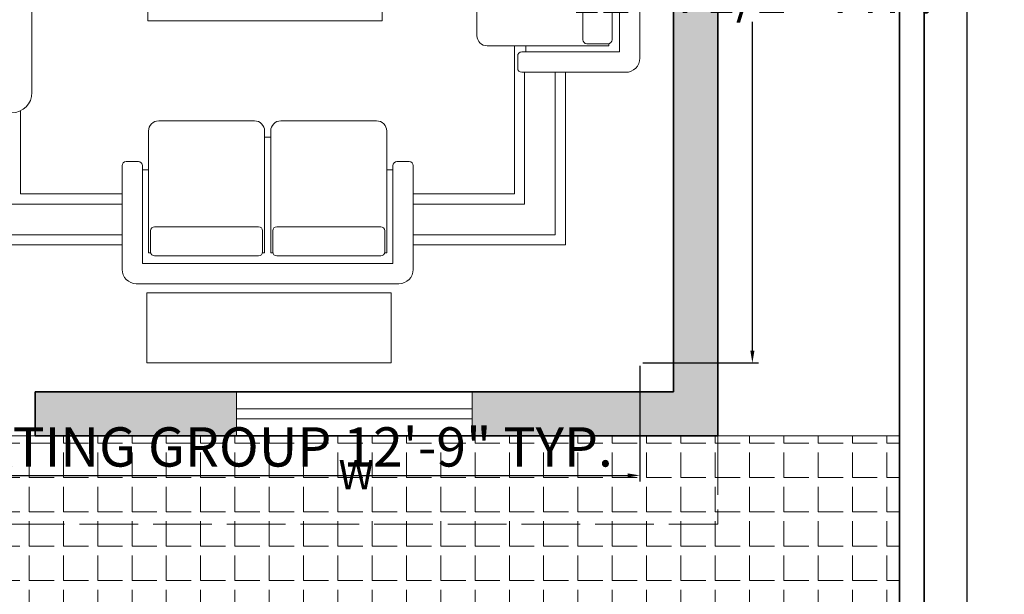
# Model space of a CAD drawing. Units: inches. Extents: x 1070 to 2371, y 645 to 1546.
# Tile 4 of 10: x 1458 to 1658, y 772 to 890. Entities that reach past the tile are written whole.
import ezdxf

# ---------------------------------------------------------------- set-up
doc = ezdxf.new("R2010")
doc.units = ezdxf.units.IN
doc.linetypes.add('ACAD_ISO02W100', pattern=[15, 12, -3])
for name, color, linetype, lineweight in [('A-ANNO-DIMS', 2, 'Continuous', 18), ('A-ANNO-TEXT', 7, 'Continuous', 18), ('A-DOOR', 4, 'Continuous', 18), ('A-FURN', 8, 'Continuous', 18), ('A-GLAZ', 4, 'Continuous', 18), ('A-ROOF-OVHD', 8, 'ACAD_ISO02W100', 13), ('A-WALL', 7, 'Continuous', 35), ('C-PROP', 7, 'Continuous', 35), ('L-PLNT-BEDS', 3, 'Continuous', 18), ('L-TURF-PATT', 9, 'Continuous', 13)]:
    doc.layers.add(name, color=color, linetype=linetype, lineweight=lineweight)
doc.layers.add('A-WALL-PATT', color=162, linetype='Continuous', lineweight=13, true_color=0x044ac3)
doc.styles.get("Standard").update_dxf_attribs({"font": 'arial.ttf'})
doc.dimstyles.new('ISO-25', dxfattribs={"dimtxt": 8, "dimasz": 2.5, "dimexe": 1.25, "dimexo": 0.625, "dimtad": 1, "dimtih": 1, "dimtoh": 1, "dimdec": 1, "dimlunit": 3, "dimtxsty": 'Standard', "dimcen": 2.5, "dimadec": 0, "dimazin": 0, "dimtfac": 1, "dimtdec": 1, "dimtmove": 0, "dimatfit": 3, "dimfxl": 1, "dimarcsym": 0})

# ---------------------------------------------------------------- blocks, each defined once
blk = doc.blocks.new('A$C71DE5BFE')
for p, q in [((2753, 3552), (893, 3552)), ((823, 3482), (823, 2972)), ((2823, 2972), (2823, 3482)), ((923, 3452), (2723, 3452)), ((923, 2972), (923, 3452)), ((2723, 3452), (2723, 2972)), ((430.7, 3295.7), (503.4, 3397.4)), ((963.5, 3399.9), (953, 3399.9)), ((953, 3399.9), (953, 2802)), ((963, 3292), (963, 3395.7)), ((1493, 3415.7), (983, 3415.7)), ((1523, 3399.9), (1512.6, 3399.9)), ((1513, 3292), (1513, 3395.7)), ((1523, 2802), (1523, 3399.9)), ((1553.5, 3399.9), (1543, 3399.9)), ((1543, 2802), (1543, 3399.9)), ((1553, 3292), (1553, 3395.7)), ((2073, 3415.7), (1573, 3415.7)), ((2103, 3399.9), (2092.6, 3399.9)), ((2093, 3292), (2093, 3395.7)), ((2103, 2802), (2103, 3399.9)), ((2133.5, 3399.9), (2123, 3399.9)), ((2123, 2802), (2123, 3399.9)), ((2133, 3292), (2133, 3395.7)), ((2663, 3415.7), (2153, 3415.7)), ((2693, 3399.9), (2683, 3399.9)), ((2683, 3292), (2683, 3395.7)), ((2693, 2802), (2693, 3399.9)), ((3215.3, 3295.7), (3142.7, 3397.4)), ((437, 3290.4), (525.4, 3378.7)), ((3209, 3290.4), (3120.6, 3378.7)), ((353.2, 3267.1), (231.9, 3297.4)), ((3292.9, 3267.1), (3414.1, 3297.4)), ((352, 3261.2), (228, 3276.7)), ((1493, 3272), (983, 3272)), ((2073, 3272), (1573, 3272)), ((2663, 3272), (2153, 3272)), ((3294, 3261.2), (3418, 3276.7)), ((426.5, 3211.6), (488.5, 3103.1)), ((430.7, 3214.3), (503.4, 3112.6)), ((3215.3, 3214.3), (3142.7, 3112.6)), ((3219.6, 3211.6), (3157.6, 3103.1)), ((726.7, 3055), (823, 3055)), ((2823, 3055), (2919.4, 3055)), ((726.7, 3005), (823, 3005)), ((2823, 3005), (2919.4, 3005)), ((843, 2952), (903, 2952)), ((953, 2992), (923, 2992)), ((2723, 2992), (2693, 2992)), ((2743, 2952), (2803, 2952)), ((394.4, 2753.9), (394.4, 2930)), ((444.4, 2753.9), (444.4, 2930)), ((3269.4, 2930), (3269.4, 2857.9)), ((3319.4, 2930), (3319.4, 2857.9)), ((2693, 2855), (3119.4, 2855)), ((3615.1, 2857.9), (3105.1, 2857.9)), ((1543, 2832), (1523, 2832)), ((2123, 2832), (2103, 2832)), ((2693, 2805), (3069.4, 2805)), ((3069.4, 2805), (3069.4, 2727.9)), ((3085.1, 2837.9), (3085.1, 2777.9)), ((3105.1, 2757.9), (3585.1, 2757.9)), ((3125.1, 2727.9), (3125.1, 2757.9)), ((3585.1, 2757.9), (3585.1, 1527.9)), ((3685.1, 1497.9), (3685.1, 2787.9)), ((350, 2753.9), (510, 2753.9)), ((540, 2723.9), (540, 2703.9)), ((1473, 2752), (1003, 2752)), ((2053, 2752), (1593, 2752)), ((2643, 2752), (2173, 2752)), ((3532.9, 2727.9), (2935.1, 2727.9)), ((3425.1, 2717.9), (3528.7, 2717.9)), ((3532.9, 2717.5), (3532.9, 2727.9)), ((202.1, 2655.3), (206.4, 2659.6)), ((206.4, 2659.6), (210.7, 2661.9)), ((210.7, 2661.9), (213.1, 2666.2)), ((213.1, 2666.2), (217.4, 2668.5)), ((217.4, 2668.5), (219.7, 2672.9)), ((219.7, 2672.9), (224, 2672.9)), ((224, 2672.9), (228.3, 2675.2)), ((228.3, 2675.2), (232.7, 2677.2)), ((232.7, 2677.2), (245.9, 2677.2)), ((245.9, 2677.2), (250.2, 2679.5)), ((250.2, 2679.5), (254.6, 2681.5)), ((254.6, 2681.5), (256.9, 2686.1)), ((256.9, 2686.1), (261.2, 2686.1)), ((261.2, 2686.1), (265.5, 2688.1)), ((265.5, 2688.1), (270.1, 2688.1)), ((270.1, 2688.1), (274.4, 2690.5)), ((272.1, 2657.6), (276.5, 2661.9)), ((274.4, 2690.5), (283.1, 2690.5)), ((276.5, 2661.9), (281.1, 2664.2)), ((281.1, 2664.2), (283.1, 2668.5)), ((283.1, 2690.5), (287.7, 2692.5)), ((283.1, 2668.5), (285.4, 2672.9)), ((285.4, 2672.9), (289.7, 2677.2)), ((287.7, 2692.5), (305, 2692.5)), ((289.7, 2677.2), (292, 2681.5)), ((292, 2659.6), (289.7, 2655.3)), ((292, 2681.5), (296.3, 2686.1)), ((296.3, 2664.2), (292, 2659.6)), ((296.3, 2686.1), (298.6, 2690.5)), ((300.7, 2668.5), (296.3, 2664.2)), ((298.6, 2690.5), (300.7, 2694.8)), ((300.7, 2694.8), (303, 2694.8)), ((305, 2675.2), (300.7, 2668.5)), ((305, 2692.5), (309.6, 2694.8)), ((309.6, 2677.2), (305, 2675.2)), ((309.6, 2694.8), (322.6, 2694.8)), ((311.6, 2681.5), (309.6, 2677.2)), ((315.9, 2683.8), (311.6, 2681.5)), ((320.5, 2686.1), (315.9, 2683.8)), ((318.2, 2697.1), (322.6, 2697.1)), ((322.6, 2690.5), (320.5, 2686.1)), ((322.6, 2694.8), (326.9, 2697.1)), ((322.6, 2697.1), (326.9, 2694.8)), ((326.9, 2694.8), (322.6, 2690.5)), ((326.9, 2697.1), (329.2, 2697.1)), ((326.9, 2694.8), (331.5, 2686.1)), ((331.5, 2686.1), (333.5, 2681.5)), ((333.5, 2681.5), (333.5, 2677.2)), ((333.5, 2677.2), (335.8, 2672.9)), ((335.8, 2659.6), (333.5, 2655.3)), ((335.8, 2672.9), (335.8, 2659.6)), ((350, 2703.9), (600, 2703.9)), ((2885.1, 2207.9), (2885.1, 2677.9)), ((3405.1, 2187.9), (3405.1, 2697.9)), ((3548.7, 2187.9), (3548.7, 2697.9)), ((138.4, 2609.4), (143, 2611.4)), ((143, 2615.7), (147.3, 2618)), ((143, 2611.4), (143, 2615.7)), ((147.3, 2618), (149.4, 2622.4)), ((149.4, 2622.4), (154, 2624.7)), ((154, 2624.7), (158.3, 2626.7)), ((158.3, 2626.7), (162.6, 2631.3)), ((162.6, 2631.3), (166.9, 2635.6)), ((166.9, 2635.6), (171.3, 2637.7)), ((171.3, 2637.7), (175.9, 2640)), ((175.9, 2640), (180.2, 2642.3)), ((180.2, 2642.3), (184.5, 2646.6)), ((184.5, 2646.6), (188.8, 2648.6)), ((188.8, 2648.6), (193.5, 2650.9)), ((193.5, 2650.9), (197.8, 2653.2)), ((197.8, 2653.2), (202.1, 2655.3)), ((239.3, 2611.4), (241.6, 2615.7)), ((239.3, 2607.1), (239.3, 2611.4)), ((241.6, 2615.7), (243.6, 2620.4)), ((243.6, 2620.4), (248.2, 2624.7)), ((248.2, 2624.7), (250.2, 2629)), ((250.2, 2629), (252.5, 2633.3)), ((252.5, 2633.3), (256.9, 2637.7)), ((256.9, 2637.7), (259.2, 2642.3)), ((259.2, 2642.3), (261.2, 2646.6)), ((261.2, 2646.6), (263.5, 2650.9)), ((263.5, 2650.9), (267.8, 2655.3)), ((267.8, 2655.3), (272.1, 2657.6)), ((272.1, 2615.7), (267.8, 2605.1)), ((276.5, 2620.4), (272.1, 2615.7)), ((281.1, 2629), (276.5, 2624.7)), ((276.5, 2624.7), (276.5, 2620.4)), ((283.1, 2633.3), (281.1, 2629)), ((285.4, 2637.7), (283.1, 2633.3)), ((287.7, 2648.6), (285.4, 2644.3)), ((285.4, 2644.3), (285.4, 2637.7)), ((289.7, 2655.3), (287.7, 2648.6)), ((318.2, 2611.4), (315.9, 2607.1)), ((320.5, 2620.4), (318.2, 2615.7)), ((318.2, 2615.7), (318.2, 2611.4)), ((322.6, 2629), (320.5, 2624.7)), ((320.5, 2624.7), (320.5, 2620.4)), ((324.9, 2633.3), (322.6, 2629)), ((329.2, 2637.7), (324.9, 2633.3)), ((331.5, 2646.6), (329.2, 2642.3)), ((329.2, 2642.3), (329.2, 2637.7)), ((333.5, 2650.9), (331.5, 2646.6)), ((333.5, 2655.3), (333.5, 2650.9)), ((99.2, 2561.2), (103.5, 2563.2)), ((103.5, 2563.2), (105.6, 2567.6)), ((105.6, 2567.6), (110.2, 2567.6)), ((110.2, 2572.2), (114.5, 2574.2)), ((110.2, 2567.6), (110.2, 2572.2)), ((114.5, 2574.2), (116.5, 2578.5)), ((116.5, 2578.5), (118.8, 2583.1)), ((118.8, 2583.1), (123.1, 2585.2)), ((123.1, 2589.5), (127.5, 2591.8)), ((123.1, 2585.2), (123.1, 2589.5)), ((127.5, 2591.8), (129.8, 2596.1)), ((129.8, 2596.1), (134.1, 2600.5)), ((134.1, 2600.5), (136.4, 2605.1)), ((136.4, 2605.1), (138.4, 2609.4)), ((226.3, 2561.2), (228.3, 2565.5)), ((228.3, 2565.5), (230.6, 2569.9)), ((230.6, 2574.2), (232.7, 2580.8)), ((230.6, 2569.9), (230.6, 2574.2)), ((232.7, 2589.5), (235, 2594.1)), ((232.7, 2580.8), (232.7, 2589.5)), ((235, 2598.4), (237.3, 2602.8)), ((235, 2594.1), (235, 2598.4)), ((237.3, 2602.8), (239.3, 2607.1)), ((243.6, 2567.6), (241.6, 2561.2)), ((248.2, 2574.2), (243.6, 2567.6)), ((250.2, 2578.5), (248.2, 2574.2)), ((254.6, 2585.2), (250.2, 2578.5)), ((259.2, 2594.1), (254.6, 2585.2)), ((267.8, 2605.1), (259.2, 2594.1)), ((298.6, 2569.9), (294, 2561.2)), ((300.7, 2578.5), (298.6, 2569.9)), ((303, 2585.2), (300.7, 2578.5)), ((311.6, 2598.4), (303, 2589.5)), ((303, 2589.5), (303, 2585.2)), ((315.9, 2607.1), (311.6, 2598.4)), ((700, 2603.9), (700, 2203.9)), ((68.4, 2510.7), (70.7, 2515.1)), ((70.7, 2515.1), (72.7, 2519.4)), ((72.7, 2519.4), (75, 2523.7)), ((75, 2523.7), (79.3, 2528.3)), ((79.3, 2528.3), (83.7, 2530.4)), ((83.7, 2530.4), (86, 2534.7)), ((86, 2534.7), (88.3, 2539.3)), ((88.3, 2539.3), (90.3, 2543.6)), ((90.3, 2543.6), (92.6, 2547.9)), ((92.6, 2547.9), (94.6, 2552.3)), ((94.6, 2552.3), (99.2, 2556.6)), ((99.2, 2556.6), (99.2, 2561.2)), ((210.7, 2515.1), (213.1, 2519.4)), ((210.7, 2510.7), (210.7, 2515.1)), ((213.1, 2519.4), (217.4, 2526)), ((217.4, 2530.4), (219.7, 2534.7)), ((217.4, 2526), (217.4, 2530.4)), ((219.7, 2541.3), (221.7, 2547.9)), ((219.7, 2534.7), (219.7, 2541.3)), ((221.7, 2552.3), (224, 2556.6)), ((221.7, 2547.9), (221.7, 2552.3)), ((224, 2556.6), (226.3, 2561.2)), ((235, 2534.7), (232.7, 2530.4)), ((232.7, 2530.4), (232.7, 2510.7)), ((237.3, 2541.3), (235, 2534.7)), ((239.3, 2552.3), (237.3, 2545.6)), ((237.3, 2545.6), (237.3, 2541.3)), ((241.6, 2561.2), (239.3, 2556.6)), ((239.3, 2556.6), (239.3, 2552.3)), ((289.7, 2528.3), (285.4, 2519.4)), ((285.4, 2519.4), (285.4, 2499.8)), ((292, 2541.3), (289.7, 2534.7)), ((289.7, 2534.7), (289.7, 2528.3)), ((294, 2556.6), (292, 2547.9)), ((292, 2547.9), (292, 2541.3)), ((294, 2561.2), (294, 2556.6)), ((57.4, 2471.2), (59.7, 2475.5)), ((57.4, 2462.6), (57.4, 2471.2)), ((59.7, 2475.5), (61.8, 2480.2)), ((61.8, 2480.2), (64.1, 2484.5)), ((64.1, 2488.8), (66.4, 2493.1)), ((64.1, 2484.5), (64.1, 2488.8)), ((66.4, 2497.5), (68.4, 2502.1)), ((66.4, 2493.1), (66.4, 2497.5)), ((68.4, 2502.1), (68.4, 2510.7)), ((204.4, 2464.6), (206.4, 2469.2)), ((206.4, 2493.1), (208.7, 2497.5)), ((206.4, 2469.2), (206.4, 2493.1)), ((208.7, 2506.4), (210.7, 2510.7)), ((208.7, 2497.5), (208.7, 2506.4)), ((217.4, 2471.2), (215.4, 2466.9)), ((215.4, 2466.9), (215.4, 2436.3)), ((219.7, 2475.5), (217.4, 2471.2)), ((221.7, 2482.2), (219.7, 2475.5)), ((224, 2486.5), (221.7, 2482.2)), ((226.3, 2491.1), (224, 2486.5)), ((228.3, 2497.5), (226.3, 2491.1)), ((230.6, 2504.1), (228.3, 2497.5)), ((232.7, 2510.7), (230.6, 2504.1)), ((285.4, 2499.8), (276.5, 2482.2)), ((276.5, 2482.2), (276.5, 2453.6)), ((55.1, 2423), (57.4, 2427.4)), ((55.1, 2405.4), (55.1, 2423)), ((59.7, 2458.2), (57.4, 2462.6)), ((57.4, 2436.3), (59.7, 2440.6)), ((57.4, 2427.4), (57.4, 2436.3)), ((59.7, 2440.6), (59.7, 2458.2)), ((193.5, 2414.4), (197.8, 2427.4)), ((197.8, 2427.4), (199.8, 2431.7)), ((199.8, 2431.7), (202.1, 2436.3)), ((202.1, 2440.6), (204.4, 2445)), ((202.1, 2436.3), (202.1, 2440.6)), ((204.4, 2445), (204.4, 2464.6)), ((215.4, 2436.3), (206.4, 2418.7)), ((206.4, 2418.7), (206.4, 2392.5)), ((267.8, 2427.4), (259.2, 2410.1)), ((276.5, 2453.6), (267.8, 2445)), ((267.8, 2445), (267.8, 2427.4)), ((53.1, 2401.1), (55.1, 2405.4)), ((53.1, 2392.5), (53.1, 2401.1)), ((55.1, 2388.1), (53.1, 2392.5)), ((55.1, 2361.6), (55.1, 2388.1)), ((184.5, 2377.2), (186.8, 2381.5)), ((184.5, 2363.9), (184.5, 2377.2)), ((186.8, 2392.5), (188.8, 2396.8)), ((186.8, 2381.5), (186.8, 2392.5)), ((188.8, 2401.1), (191.2, 2405.4)), ((188.8, 2396.8), (188.8, 2401.1)), ((191.2, 2405.4), (193.5, 2414.4)), ((197.8, 2372.6), (195.5, 2368.2)), ((206.4, 2392.5), (197.8, 2383.5)), ((197.8, 2383.5), (197.8, 2372.6)), ((250.2, 2370.5), (248.2, 2366.2)), ((259.2, 2392.5), (250.2, 2374.9)), ((250.2, 2374.9), (250.2, 2370.5)), ((259.2, 2410.1), (259.2, 2392.5)), ((57.4, 2357.3), (55.1, 2361.6)), ((57.4, 2352.9), (57.4, 2357.3)), ((59.7, 2348.6), (57.4, 2352.9)), ((59.7, 2344.3), (59.7, 2348.6)), ((61.8, 2340), (59.7, 2344.3)), ((64.1, 2335.3), (61.8, 2340)), ((66.4, 2331), (64.1, 2335.3)), ((66.4, 2326.7), (66.4, 2331)), ((68.4, 2322.4), (66.4, 2326.7)), ((68.4, 2318), (68.4, 2322.4)), ((175.9, 2315.7), (177.9, 2322.4)), ((177.9, 2335.3), (180.2, 2342)), ((177.9, 2322.4), (177.9, 2335.3)), ((180.2, 2350.6), (182.5, 2357.3)), ((180.2, 2342), (180.2, 2350.6)), ((182.5, 2357.3), (184.5, 2363.9)), ((195.5, 2363.9), (193.5, 2359.6)), ((193.5, 2359.6), (193.5, 2274.2)), ((195.5, 2368.2), (195.5, 2363.9)), ((248.2, 2366.2), (248.2, 2307.1)), ((70.7, 2311.4), (68.4, 2318)), ((72.7, 2307.1), (70.7, 2311.4)), ((75, 2302.5), (72.7, 2307.1)), ((77.3, 2298.1), (75, 2302.5)), ((77.3, 2293.8), (77.3, 2298.1)), ((79.3, 2289.5), (77.3, 2293.8)), ((81.6, 2285.1), (79.3, 2289.5)), ((83.7, 2278.5), (81.6, 2285.1)), ((86, 2274.2), (83.7, 2278.5)), ((88.3, 2269.6), (86, 2274.2)), ((175.9, 2311.4), (175.9, 2315.7)), ((177.9, 2307.1), (175.9, 2311.4)), ((177.9, 2298.1), (177.9, 2307.1)), ((180.2, 2293.8), (177.9, 2298.1)), ((180.2, 2254.3), (180.2, 2293.8)), ((193.5, 2274.2), (195.5, 2265.2)), ((248.2, 2307.1), (245.9, 2300.4)), ((245.9, 2300.4), (245.9, 2263.2)), ((90.3, 2265.2), (88.3, 2269.6)), ((94.6, 2263.2), (90.3, 2265.2)), ((96.9, 2258.6), (94.6, 2263.2)), ((101.2, 2256.6), (96.9, 2258.6)), ((103.5, 2252.3), (101.2, 2256.6)), ((107.9, 2250), (103.5, 2252.3)), ((112.2, 2245.6), (107.9, 2250)), ((121.1, 2239), (112.2, 2245.6)), ((134.1, 2226), (121.1, 2239)), ((136.4, 2221.4), (134.1, 2226)), ((182.5, 2250), (180.2, 2254.3)), ((182.5, 2245.6), (182.5, 2250)), ((184.5, 2239), (182.5, 2245.6)), ((184.5, 2212.7), (184.5, 2239)), ((195.5, 2265.2), (195.5, 2252.3)), ((195.5, 2252.3), (197.8, 2247.9)), ((197.8, 2247.9), (197.8, 2243.3)), ((197.8, 2243.3), (199.8, 2232.4)), ((199.8, 2232.4), (199.8, 2215)), ((243.6, 2228), (241.6, 2223.7)), ((245.9, 2237), (243.6, 2232.4)), ((243.6, 2232.4), (243.6, 2228)), ((245.9, 2263.2), (248.2, 2258.6)), ((248.2, 2241.3), (245.9, 2237)), ((248.2, 2258.6), (248.2, 2241.3)), ((140.7, 2219.4), (136.4, 2221.4)), ((143, 2215), (140.7, 2219.4)), ((145, 2210.4), (143, 2215)), ((147.3, 2206.1), (145, 2210.4)), ((149.4, 2201.8), (147.3, 2206.1)), ((151.7, 2197.5), (149.4, 2201.8)), ((154, 2190.8), (151.7, 2197.5)), ((154, 2186.5), (154, 2190.8)), ((156, 2182.2), (154, 2186.5)), ((160.3, 2179.9), (156, 2182.2)), ((162.6, 2175.5), (160.3, 2179.9)), ((186.8, 2208.4), (184.5, 2212.7)), ((186.8, 2204.1), (186.8, 2208.4)), ((188.8, 2199.5), (186.8, 2204.1)), ((188.8, 2190.8), (188.8, 2199.5)), ((191.2, 2186.5), (188.8, 2190.8)), ((191.2, 2179.9), (191.2, 2186.5)), ((193.5, 2175.5), (191.2, 2179.9)), ((199.8, 2215), (202.1, 2208.4)), ((202.1, 2208.4), (202.1, 2186.5)), ((202.1, 2186.5), (204.4, 2182.2)), ((204.4, 2182.2), (204.4, 2173.2)), ((239.3, 2184.2), (237.3, 2179.9)), ((237.3, 2179.9), (237.3, 2175.5)), ((241.6, 2197.5), (239.3, 2193.1)), ((239.3, 2193.1), (239.3, 2184.2)), ((241.6, 2223.7), (241.6, 2197.5)), ((166.9, 2171.2), (162.6, 2175.5)), ((169.2, 2166.6), (166.9, 2171.2)), ((173.6, 2166.6), (169.2, 2166.6)), ((175.9, 2162.3), (173.6, 2166.6)), ((180.2, 2162.3), (175.9, 2162.3)), ((184.5, 2160.2), (180.2, 2162.3)), ((188.8, 2157.9), (184.5, 2160.2)), ((195.5, 2153.6), (188.8, 2157.9)), ((195.5, 2171.2), (193.5, 2175.5)), ((195.5, 2162.3), (195.5, 2171.2)), ((197.8, 2157.9), (195.5, 2162.3)), ((199.8, 2151.3), (195.5, 2153.6)), ((199.8, 2153.6), (197.8, 2157.9)), ((199.8, 2149.3), (199.8, 2153.6)), ((204.4, 2149.3), (199.8, 2151.3)), ((204.4, 2173.2), (206.4, 2168.9)), ((208.7, 2147), (204.4, 2149.3)), ((206.4, 2168.9), (206.4, 2164.6)), ((206.4, 2164.6), (208.7, 2160.2)), ((208.7, 2160.2), (210.7, 2155.9)), ((213.1, 2149.3), (208.7, 2147)), ((210.7, 2155.9), (213.1, 2151.3)), ((213.1, 2151.3), (213.1, 2149.3)), ((226.3, 2149.3), (213.1, 2149.3)), ((228.3, 2153.6), (226.3, 2149.3)), ((232.7, 2157.9), (228.3, 2153.6)), ((235, 2162.3), (232.7, 2157.9)), ((237.3, 2175.5), (235, 2171.2)), ((235, 2171.2), (235, 2162.3)), ((2935.1, 2157.9), (3532.9, 2157.9)), ((2935.1, 2127.9), (3532.9, 2127.9)), ((2965.1, 2137.9), (2965.1, 2157.9)), ((2965.1, 2127.9), (2965.1, 2147.9)), ((3425.1, 2167.9), (3528.7, 2167.9)), ((3532.9, 2157.9), (3532.9, 2168.4)), ((3532.9, 2117.5), (3532.9, 2127.9)), ((350, 2103.9), (600, 2103.9)), ((540, 2103.9), (540, 2083.9)), ((594.4, 1828.9), (594.4, 2103.9)), ((644.4, 1818.6), (644.4, 2114.3)), ((3405.1, 1587.9), (3405.1, 2097.9)), ((3425.1, 2117.9), (3528.7, 2117.9)), ((3548.7, 1587.9), (3548.7, 2097.9)), ((510, 2053.9), (350, 2053.9)), ((394.4, 1878.9), (394.4, 2053.9)), ((444.4, 1878.9), (444.4, 2053.9)), ((2885.1, 1607.9), (2885.1, 2077.9)), ((350, 1878.9), (510, 1878.9)), ((540, 1848.9), (540, 1828.9)), ((210.7, 1786.9), (213.1, 1791.2)), ((213.1, 1791.2), (217.4, 1793.5)), ((217.4, 1793.5), (219.7, 1797.9)), ((219.7, 1797.9), (224, 1797.9)), ((224, 1797.9), (228.3, 1800.2)), ((228.3, 1800.2), (232.7, 1802.2)), ((232.7, 1802.2), (245.9, 1802.2)), ((245.9, 1802.2), (250.2, 1804.5)), ((250.2, 1804.5), (254.6, 1806.5)), ((254.6, 1806.5), (256.9, 1811.1)), ((256.9, 1811.1), (261.2, 1811.1)), ((261.2, 1811.1), (265.5, 1813.1)), ((265.5, 1813.1), (270.1, 1813.1)), ((270.1, 1813.1), (274.4, 1815.5)), ((274.4, 1815.5), (283.1, 1815.5)), ((276.5, 1786.9), (281.1, 1789.2)), ((281.1, 1789.2), (283.1, 1793.5)), ((283.1, 1815.5), (287.7, 1817.5)), ((283.1, 1793.5), (285.4, 1797.9)), ((285.4, 1797.9), (289.7, 1802.2)), ((287.7, 1817.5), (305, 1817.5)), ((289.7, 1802.2), (292, 1806.5)), ((292, 1806.5), (296.3, 1811.1)), ((296.3, 1789.2), (292, 1784.6)), ((296.3, 1811.1), (298.6, 1815.5)), ((300.7, 1793.5), (296.3, 1789.2)), ((298.6, 1815.5), (300.7, 1819.8)), ((300.7, 1819.8), (303, 1819.8)), ((305, 1800.2), (300.7, 1793.5)), ((305, 1817.5), (309.6, 1819.8)), ((309.6, 1802.2), (305, 1800.2)), ((309.6, 1819.8), (322.6, 1819.8)), ((311.6, 1806.5), (309.6, 1802.2)), ((315.9, 1808.8), (311.6, 1806.5)), ((320.5, 1811.1), (315.9, 1808.8)), ((318.2, 1822.1), (322.6, 1822.1)), ((322.6, 1815.5), (320.5, 1811.1)), ((322.6, 1819.8), (326.9, 1822.1)), ((322.6, 1822.1), (326.9, 1819.8)), ((326.9, 1819.8), (322.6, 1815.5)), ((326.9, 1822.1), (329.2, 1822.1)), ((326.9, 1819.8), (331.5, 1811.1)), ((331.5, 1811.1), (333.5, 1806.5)), ((333.5, 1806.5), (333.5, 1802.2)), ((333.5, 1802.2), (335.8, 1797.9)), ((335.8, 1797.9), (335.8, 1784.6)), ((350, 1828.9), (600, 1828.9)), ((143, 1740.7), (147.3, 1743)), ((143, 1736.4), (143, 1740.7)), ((147.3, 1743), (149.4, 1747.4)), ((149.4, 1747.4), (154, 1749.7)), ((154, 1749.7), (158.3, 1751.7)), ((158.3, 1751.7), (162.6, 1756.3)), ((162.6, 1756.3), (166.9, 1760.6)), ((166.9, 1760.6), (171.3, 1762.7)), ((171.3, 1762.7), (175.9, 1765)), ((175.9, 1765), (180.2, 1767.3)), ((180.2, 1767.3), (184.5, 1771.6)), ((184.5, 1771.6), (188.8, 1773.6)), ((188.8, 1773.6), (193.5, 1775.9)), ((193.5, 1775.9), (197.8, 1778.2)), ((197.8, 1778.2), (202.1, 1780.3)), ((202.1, 1780.3), (206.4, 1784.6)), ((206.4, 1784.6), (210.7, 1786.9)), ((239.3, 1736.4), (241.6, 1740.7)), ((241.6, 1740.7), (243.6, 1745.4)), ((243.6, 1745.4), (248.2, 1749.7)), ((248.2, 1749.7), (250.2, 1754)), ((250.2, 1754), (252.5, 1758.3)), ((252.5, 1758.3), (256.9, 1762.7)), ((256.9, 1762.7), (259.2, 1767.3)), ((259.2, 1767.3), (261.2, 1771.6)), ((261.2, 1771.6), (263.5, 1775.9)), ((263.5, 1775.9), (267.8, 1780.3)), ((267.8, 1780.3), (272.1, 1782.6)), ((272.1, 1740.7), (267.8, 1730.1)), ((272.1, 1782.6), (276.5, 1786.9)), ((276.5, 1745.4), (272.1, 1740.7)), ((281.1, 1754), (276.5, 1749.7)), ((276.5, 1749.7), (276.5, 1745.4)), ((283.1, 1758.3), (281.1, 1754)), ((285.4, 1762.7), (283.1, 1758.3)), ((287.7, 1773.6), (285.4, 1769.3)), ((285.4, 1769.3), (285.4, 1762.7)), ((289.7, 1780.3), (287.7, 1773.6)), ((292, 1784.6), (289.7, 1780.3)), ((320.5, 1745.4), (318.2, 1740.7)), ((318.2, 1740.7), (318.2, 1736.4)), ((322.6, 1754), (320.5, 1749.7)), ((320.5, 1749.7), (320.5, 1745.4)), ((324.9, 1758.3), (322.6, 1754)), ((329.2, 1762.7), (324.9, 1758.3)), ((331.5, 1771.6), (329.2, 1767.3)), ((329.2, 1767.3), (329.2, 1762.7)), ((333.5, 1775.9), (331.5, 1771.6)), ((335.8, 1784.6), (333.5, 1780.3)), ((333.5, 1780.3), (333.5, 1775.9)), ((103.5, 1688.2), (105.6, 1692.6)), ((105.6, 1692.6), (110.2, 1692.6)), ((110.2, 1697.2), (114.5, 1699.2)), ((110.2, 1692.6), (110.2, 1697.2)), ((114.5, 1699.2), (116.5, 1703.5)), ((116.5, 1703.5), (118.8, 1708.1)), ((118.8, 1708.1), (123.1, 1710.2)), ((123.1, 1714.5), (127.5, 1716.8)), ((123.1, 1710.2), (123.1, 1714.5)), ((127.5, 1716.8), (129.8, 1721.1)), ((129.8, 1721.1), (134.1, 1725.5)), ((134.1, 1725.5), (136.4, 1730.1)), ((136.4, 1730.1), (138.4, 1734.4)), ((138.4, 1734.4), (143, 1736.4)), ((228.3, 1690.5), (230.6, 1694.9)), ((230.6, 1699.2), (232.7, 1705.8)), ((230.6, 1694.9), (230.6, 1699.2)), ((232.7, 1714.5), (235, 1719.1)), ((232.7, 1705.8), (232.7, 1714.5)), ((235, 1723.4), (237.3, 1727.8)), ((235, 1719.1), (235, 1723.4)), ((237.3, 1727.8), (239.3, 1732.1)), ((239.3, 1732.1), (239.3, 1736.4)), ((243.6, 1692.6), (241.6, 1686.2)), ((248.2, 1699.2), (243.6, 1692.6)), ((250.2, 1703.5), (248.2, 1699.2)), ((254.6, 1710.2), (250.2, 1703.5)), ((259.2, 1719.1), (254.6, 1710.2)), ((267.8, 1730.1), (259.2, 1719.1)), ((298.6, 1694.9), (294, 1686.2)), ((300.7, 1703.5), (298.6, 1694.9)), ((303, 1710.2), (300.7, 1703.5)), ((311.6, 1723.4), (303, 1714.5)), ((303, 1714.5), (303, 1710.2)), ((315.9, 1732.1), (311.6, 1723.4)), ((318.2, 1736.4), (315.9, 1732.1)), ((700, 1728.9), (700, 1328.9)), ((70.7, 1640.1), (72.7, 1644.4)), ((72.7, 1644.4), (75, 1648.7)), ((75, 1648.7), (79.3, 1653.3)), ((79.3, 1653.3), (83.7, 1655.4)), ((83.7, 1655.4), (86, 1659.7)), ((86, 1659.7), (88.3, 1664.3)), ((88.3, 1664.3), (90.3, 1668.6)), ((90.3, 1668.6), (92.6, 1672.9)), ((92.6, 1672.9), (94.6, 1677.3)), ((94.6, 1677.3), (99.2, 1681.6)), ((99.2, 1686.2), (103.5, 1688.2)), ((99.2, 1681.6), (99.2, 1686.2)), ((210.7, 1640.1), (213.1, 1644.4)), ((213.1, 1644.4), (217.4, 1651)), ((217.4, 1655.4), (219.7, 1659.7)), ((217.4, 1651), (217.4, 1655.4)), ((219.7, 1666.3), (221.7, 1672.9)), ((219.7, 1659.7), (219.7, 1666.3)), ((221.7, 1677.3), (224, 1681.6)), ((221.7, 1672.9), (221.7, 1677.3)), ((224, 1681.6), (226.3, 1686.2)), ((226.3, 1686.2), (228.3, 1690.5)), ((235, 1659.7), (232.7, 1655.4)), ((232.7, 1655.4), (232.7, 1635.7)), ((237.3, 1666.3), (235, 1659.7)), ((239.3, 1677.3), (237.3, 1670.6)), ((237.3, 1670.6), (237.3, 1666.3)), ((241.6, 1686.2), (239.3, 1681.6)), ((239.3, 1681.6), (239.3, 1677.3)), ((289.7, 1653.3), (285.4, 1644.4)), ((285.4, 1644.4), (285.4, 1624.8)), ((292, 1666.3), (289.7, 1659.7)), ((289.7, 1659.7), (289.7, 1653.3)), ((294, 1681.6), (292, 1672.9)), ((292, 1672.9), (292, 1666.3)), ((294, 1686.2), (294, 1681.6)), ((57.4, 1596.2), (59.7, 1600.5)), ((57.4, 1587.6), (57.4, 1596.2)), ((59.7, 1600.5), (61.8, 1605.2)), ((61.8, 1605.2), (64.1, 1609.5)), ((64.1, 1613.8), (66.4, 1618.1)), ((64.1, 1609.5), (64.1, 1613.8)), ((66.4, 1622.5), (68.4, 1627.1)), ((66.4, 1618.1), (66.4, 1622.5)), ((68.4, 1635.7), (70.7, 1640.1)), ((68.4, 1627.1), (68.4, 1635.7)), ((206.4, 1618.1), (208.7, 1622.5)), ((206.4, 1594.2), (206.4, 1618.1)), ((208.7, 1631.4), (210.7, 1635.7)), ((208.7, 1622.5), (208.7, 1631.4)), ((210.7, 1635.7), (210.7, 1640.1)), ((217.4, 1596.2), (215.4, 1591.9)), ((219.7, 1600.5), (217.4, 1596.2)), ((221.7, 1607.2), (219.7, 1600.5)), ((224, 1611.5), (221.7, 1607.2)), ((226.3, 1616.1), (224, 1611.5)), ((228.3, 1622.5), (226.3, 1616.1)), ((230.6, 1629.1), (228.3, 1622.5)), ((232.7, 1635.7), (230.6, 1629.1)), ((285.4, 1624.8), (276.5, 1607.2)), ((276.5, 1607.2), (276.5, 1578.6)), ((55.1, 1548), (57.4, 1552.4)), ((55.1, 1530.4), (55.1, 1548)), ((59.7, 1583.2), (57.4, 1587.6)), ((57.4, 1561.3), (59.7, 1565.6)), ((57.4, 1552.4), (57.4, 1561.3)), ((59.7, 1565.6), (59.7, 1583.2)), ((193.5, 1539.4), (197.8, 1552.4)), ((197.8, 1552.4), (199.8, 1556.7)), ((199.8, 1556.7), (202.1, 1561.3)), ((202.1, 1565.6), (204.4, 1570)), ((202.1, 1561.3), (202.1, 1565.6)), ((204.4, 1589.6), (206.4, 1594.2)), ((204.4, 1570), (204.4, 1589.6)), ((215.4, 1561.3), (206.4, 1543.7)), ((215.4, 1591.9), (215.4, 1561.3)), ((267.8, 1552.4), (259.2, 1535.1)), ((276.5, 1578.6), (267.8, 1570)), ((267.8, 1570), (267.8, 1552.4)), ((2935.1, 1557.9), (3532.9, 1557.9)), ((3125.1, 1527.9), (3125.1, 1557.9)), ((3425.1, 1567.9), (3528.7, 1567.9)), ((3532.9, 1557.9), (3532.9, 1567.9)), ((53.1, 1526.1), (55.1, 1530.4)), ((53.1, 1517.5), (53.1, 1526.1)), ((55.1, 1513.1), (53.1, 1517.5)), ((55.1, 1486.6), (55.1, 1513.1)), ((184.5, 1502.2), (186.8, 1506.5)), ((184.5, 1488.9), (184.5, 1502.2)), ((186.8, 1517.5), (188.8, 1521.8)), ((186.8, 1506.5), (186.8, 1517.5)), ((188.8, 1526.1), (191.2, 1530.4)), ((188.8, 1521.8), (188.8, 1526.1)), ((191.2, 1530.4), (193.5, 1539.4)), ((206.4, 1517.5), (197.8, 1508.5)), ((197.8, 1508.5), (197.8, 1497.6)), ((206.4, 1543.7), (206.4, 1517.5)), ((259.2, 1517.5), (250.2, 1499.9)), ((250.2, 1499.9), (250.2, 1495.5)), ((259.2, 1535.1), (259.2, 1517.5)), ((3085.1, 1507.9), (3085.1, 1447.9)), ((3585.1, 1527.9), (3105.1, 1527.9)), ((57.4, 1482.3), (55.1, 1486.6)), ((57.4, 1477.9), (57.4, 1482.3)), ((59.7, 1473.6), (57.4, 1477.9)), ((59.7, 1469.3), (59.7, 1473.6)), ((61.8, 1465), (59.7, 1469.3)), ((64.1, 1460.3), (61.8, 1465)), ((66.4, 1456), (64.1, 1460.3)), ((66.4, 1451.7), (66.4, 1456)), ((68.4, 1447.4), (66.4, 1451.7)), ((177.9, 1460.3), (180.2, 1467)), ((177.9, 1447.4), (177.9, 1460.3)), ((180.2, 1475.6), (182.5, 1482.3)), ((180.2, 1467), (180.2, 1475.6)), ((182.5, 1482.3), (184.5, 1488.9)), ((195.5, 1488.9), (193.5, 1484.6)), ((193.5, 1484.6), (193.5, 1399.2)), ((197.8, 1497.6), (195.5, 1493.2)), ((195.5, 1493.2), (195.5, 1488.9)), ((250.2, 1495.5), (248.2, 1491.2)), ((248.2, 1491.2), (248.2, 1432.1)), ((68.4, 1443), (68.4, 1447.4)), ((70.7, 1436.4), (68.4, 1443)), ((72.7, 1432.1), (70.7, 1436.4)), ((75, 1427.5), (72.7, 1432.1)), ((77.3, 1423.1), (75, 1427.5)), ((77.3, 1418.8), (77.3, 1423.1)), ((79.3, 1414.5), (77.3, 1418.8)), ((81.6, 1410.1), (79.3, 1414.5)), ((83.7, 1403.5), (81.6, 1410.1)), ((86, 1399.2), (83.7, 1403.5)), ((175.9, 1440.7), (177.9, 1447.4)), ((175.9, 1436.4), (175.9, 1440.7)), ((177.9, 1432.1), (175.9, 1436.4)), ((177.9, 1423.1), (177.9, 1432.1)), ((180.2, 1418.8), (177.9, 1423.1)), ((180.2, 1379.3), (180.2, 1418.8)), ((248.2, 1432.1), (245.9, 1425.4)), ((245.9, 1425.4), (245.9, 1388.2)), ((3105.1, 1427.9), (3615.1, 1427.9)), ((88.3, 1394.6), (86, 1399.2)), ((90.3, 1390.2), (88.3, 1394.6)), ((94.6, 1388.2), (90.3, 1390.2)), ((96.9, 1383.6), (94.6, 1388.2)), ((101.2, 1381.6), (96.9, 1383.6)), ((103.5, 1377.3), (101.2, 1381.6)), ((107.9, 1375), (103.5, 1377.3)), ((112.2, 1370.6), (107.9, 1375)), ((121.1, 1364), (112.2, 1370.6)), ((134.1, 1351), (121.1, 1364)), ((182.5, 1375), (180.2, 1379.3)), ((182.5, 1370.6), (182.5, 1375)), ((184.5, 1364), (182.5, 1370.6)), ((184.5, 1337.7), (184.5, 1364)), ((193.5, 1399.2), (195.5, 1390.2)), ((195.5, 1390.2), (195.5, 1377.3)), ((195.5, 1377.3), (197.8, 1372.9)), ((197.8, 1372.9), (197.8, 1368.3)), ((197.8, 1368.3), (199.8, 1357.4)), ((199.8, 1357.4), (199.8, 1340)), ((245.9, 1362), (243.6, 1357.4)), ((243.6, 1357.4), (243.6, 1353)), ((245.9, 1388.2), (248.2, 1383.6)), ((248.2, 1366.3), (245.9, 1362)), ((248.2, 1383.6), (248.2, 1366.3)), ((136.4, 1346.4), (134.1, 1351)), ((140.7, 1344.4), (136.4, 1346.4)), ((143, 1340), (140.7, 1344.4)), ((145, 1335.4), (143, 1340)), ((147.3, 1331.1), (145, 1335.4)), ((149.4, 1326.8), (147.3, 1331.1)), ((151.7, 1322.5), (149.4, 1326.8)), ((154, 1315.8), (151.7, 1322.5)), ((154, 1311.5), (154, 1315.8)), ((156, 1307.2), (154, 1311.5)), ((160.3, 1304.9), (156, 1307.2)), ((186.8, 1333.4), (184.5, 1337.7)), ((186.8, 1329.1), (186.8, 1333.4)), ((188.8, 1324.5), (186.8, 1329.1)), ((188.8, 1315.8), (188.8, 1324.5)), ((191.2, 1311.5), (188.8, 1315.8)), ((191.2, 1304.9), (191.2, 1311.5)), ((199.8, 1340), (202.1, 1333.4)), ((202.1, 1333.4), (202.1, 1311.5)), ((202.1, 1311.5), (204.4, 1307.2)), ((204.4, 1307.2), (204.4, 1298.2)), ((239.3, 1309.2), (237.3, 1304.9)), ((241.6, 1322.5), (239.3, 1318.1)), ((239.3, 1318.1), (239.3, 1309.2)), ((243.6, 1353), (241.6, 1348.7)), ((241.6, 1348.7), (241.6, 1322.5)), ((162.6, 1300.5), (160.3, 1304.9)), ((166.9, 1296.2), (162.6, 1300.5)), ((169.2, 1291.6), (166.9, 1296.2)), ((173.6, 1291.6), (169.2, 1291.6)), ((175.9, 1287.3), (173.6, 1291.6)), ((180.2, 1287.3), (175.9, 1287.3)), ((184.5, 1285.2), (180.2, 1287.3)), ((188.8, 1282.9), (184.5, 1285.2)), ((195.5, 1278.6), (188.8, 1282.9)), ((193.5, 1300.5), (191.2, 1304.9)), ((195.5, 1296.2), (193.5, 1300.5)), ((195.5, 1287.3), (195.5, 1296.2)), ((197.8, 1282.9), (195.5, 1287.3)), ((199.8, 1276.3), (195.5, 1278.6)), ((199.8, 1278.6), (197.8, 1282.9)), ((199.8, 1274.3), (199.8, 1278.6)), ((204.4, 1274.3), (199.8, 1276.3)), ((204.4, 1298.2), (206.4, 1293.9)), ((208.7, 1272), (204.4, 1274.3)), ((206.4, 1293.9), (206.4, 1289.6)), ((206.4, 1289.6), (208.7, 1285.2)), ((208.7, 1285.2), (210.7, 1280.9)), ((213.1, 1274.3), (208.7, 1272)), ((210.7, 1280.9), (213.1, 1276.3)), ((213.1, 1276.3), (213.1, 1274.3)), ((226.3, 1274.3), (213.1, 1274.3)), ((228.3, 1278.6), (226.3, 1274.3)), ((232.7, 1282.9), (228.3, 1278.6)), ((235, 1287.3), (232.7, 1282.9)), ((237.3, 1300.5), (235, 1296.2)), ((235, 1296.2), (235, 1287.3)), ((237.3, 1304.9), (237.3, 1300.5)), ((350, 1228.9), (600, 1228.9)), ((540, 1228.9), (540, 1208.9)), ((510, 1178.9), (350, 1178.9)), ((1322.3, 1189.3), (1792.3, 1189.3)), ((1922.3, 1189.3), (2392.3, 1189.3)), ((1272.3, 1139.3), (1272.3, 541.4)), ((1842.3, 1139.3), (1842.3, 541.4)), ((1872.3, 1139.3), (1872.3, 541.4)), ((2442.3, 541.4), (2442.3, 1139.3)), ((1842.3, 1109.3), (1862.3, 1109.3)), ((1852.3, 1109.3), (1872.3, 1109.3)), ((1142.3, 969.3), (1142.3, 459.3)), ((1222.3, 989.3), (1162.3, 989.3)), ((1242.3, 489.3), (1242.3, 969.3)), ((2472.3, 969.3), (2472.3, 489.3)), ((2552.3, 989.3), (2492.3, 989.3)), ((2572.3, 459.3), (2572.3, 969.3)), ((1242.3, 949.3), (1272.3, 949.3)), ((2442.3, 949.3), (2472.3, 949.3)), ((1282.3, 649.3), (1282.3, 545.6)), ((1302.3, 669.3), (1812.3, 669.3)), ((1832.3, 649.3), (1832.3, 545.6)), ((1882.3, 649.3), (1882.3, 545.6)), ((1902.3, 669.3), (2412.3, 669.3)), ((2432.3, 649.3), (2432.3, 545.6)), ((1272.3, 541.4), (1282.3, 541.4)), ((1831.9, 541.4), (1842.3, 541.4)), ((1872.3, 541.4), (1882.7, 541.4)), ((2431.9, 541.4), (2442.3, 541.4)), ((2472.3, 489.3), (1242.3, 489.3)), ((1302.3, 525.6), (1812.3, 525.6)), ((1902.3, 525.6), (2412.3, 525.6)), ((1212.3, 389.3), (2502.3, 389.3))]:
    blk.add_line(p, q)
for points in [[(726.7, 2930), (76.7, 2930), (76.7, 3580), (726.7, 3580)], [(2919.4, 2930), (3569.4, 2930), (3569.4, 3580), (2919.4, 3580)], [(2419.4, 1680), (2419.4, 2330), (1269.4, 2330), (1269.4, 1680)], [(2464.4, 0), (2464.4, 345), (1264.4, 345), (1264.4, 0)]]:
    blk.add_lwpolyline(points, close=True)
for points in [[(594.4, 2703.9), (594.4, 2855), (953, 2855)], [(644.4, 2693.6), (644.4, 2805), (953, 2805)], [(3069.4, 1557.9), (3069.4, 830), (2572.3, 830)], [(3269.4, 1427.9), (3269.4, 630), (2572.3, 630)], [(3319.4, 1427.9), (3319.4, 580), (2572.3, 580)], [(3119.4, 1427.9), (3119.4, 780), (2572.3, 780)], [(1142.3, 780), (594.4, 780), (594.4, 1228.9)], [(1142.3, 830), (644.4, 830), (644.4, 1239.3)], [(1142.3, 580), (394.4, 580), (394.4, 1178.9)], [(1142.3, 630), (444.4, 630), (444.4, 1178.9)]]:
    blk.add_lwpolyline(points)
for centre, radius in [((401.7, 3255), 175), ((3244.4, 3255), 175), ((401.7, 3255), 50), ((3244.4, 3255), 50), ((401.7, 3255), 25), ((3244.4, 3255), 25)]:
    blk.add_circle(centre, radius)
for centre, radius, start, end in [((893, 3482), 70, 90, 180), ((2753, 3482), 70, 0, 90), ((983, 3395.7), 20, 90, 180), ((1493, 3395.7), 20, 0, 90), ((1573, 3395.7), 20, 90, 180), ((2073, 3395.7), 20, 0, 90), ((2153, 3395.7), 20, 90, 180), ((2663, 3395.7), 20, 0, 90), ((983, 3292), 20, 180, 270), ((1493, 3292), 20, 270, 0), ((1573, 3292), 20, 180, 270), ((2073, 3292), 20, 270, 0), ((2153, 3292), 20, 180, 270), ((2663, 3292), 20, 270, 0), ((843, 2972), 20, 180, 270), ((903, 2972), 20, 270, 0), ((2743, 2972), 20, 180, 270), ((2803, 2972), 20, 270, 0), ((3105.1, 2837.9), 20, 90, 180), ((3615.1, 2787.9), 70, 0, 90), ((1003, 2802), 50, 180, 270), ((1473, 2802), 50, 270, 0), ((1593, 2802), 50, 180, 270), ((2053, 2802), 50, 270, 0), ((2173, 2802), 50, 180, 270), ((2643, 2802), 50, 270, 0), ((3105.1, 2777.9), 20, 180, 270), ((350, 2403.9), 350, 90, 270), ((510, 2723.9), 30, 0, 90), ((2935.1, 2677.9), 50, 90, 180), ((3425.1, 2697.9), 20, 90, 180), ((3528.7, 2697.9), 20, 0, 90), ((350, 2403.9), 300, 90, 270), ((600, 2603.9), 100, 0, 90), ((600, 2203.9), 100, 270, 0), ((2935.1, 2207.9), 50, 180, 270), ((3425.1, 2187.9), 20, 180, 270), ((3528.7, 2187.9), 20, 270, 0), ((2935.1, 2077.9), 50, 90, 180), ((510, 2083.9), 30, 270, 0), ((3425.1, 2097.9), 20, 90, 180), ((3528.7, 2097.9), 20, 0, 90), ((350, 1528.9), 350, 90, 270), ((510, 1848.9), 30, 0, 90), ((350, 1528.9), 300, 90, 270), ((600, 1728.9), 100, 0, 90), ((2935.1, 1607.9), 50, 180, 270), ((3425.1, 1587.9), 20, 180, 270), ((3528.7, 1587.9), 20, 270, 0), ((3105.1, 1507.9), 20, 90, 180), ((3615.1, 1497.9), 70, 270, 0), ((3105.1, 1447.9), 20, 180, 270), ((600, 1328.9), 100, 270, 0), ((510, 1208.9), 30, 270, 0), ((1322.3, 1139.3), 50, 90, 180), ((1792.3, 1139.3), 50, 0, 90), ((1922.3, 1139.3), 50, 90, 180), ((2392.3, 1139.3), 50, 0, 90), ((1162.3, 969.3), 20, 90, 180), ((1222.3, 969.3), 20, 0, 90), ((2492.3, 969.3), 20, 90, 180), ((2552.3, 969.3), 20, 0, 90), ((1302.3, 649.3), 20, 90, 180), ((1812.3, 649.3), 20, 0, 90), ((1902.3, 649.3), 20, 90, 180), ((2412.3, 649.3), 20, 0, 90), ((1302.3, 545.6), 20, 180, 270), ((1812.3, 545.6), 20, 270, 0), ((1902.3, 545.6), 20, 180, 270), ((2412.3, 545.6), 20, 270, 0), ((1212.3, 459.3), 70, 180, 270), ((2502.3, 459.3), 70, 270, 0)]:
    blk.add_arc(centre, radius, start, end)
blk = doc.blocks.new('*D12')
at = {"layer": 'A-ANNO-DIMS', "color": 0, "lineweight": -2, "transparency": 16777216}
for p, q in [((1642.74, 1408.77), (1652.12, 1408.77)), ((1650.87, 1406.27), (1650.87, 1053.48)), ((1650.87, 691.27), (1650.87, 1044.06)), ((1642.74, 688.77), (1652.12, 688.77))]:
    blk.add_line(p, q, dxfattribs=at)
at = {"layer": 'A-ANNO-DIMS', "color": 0, "transparency": 16777216}
for points in [[(1650.46, 1406.27), (1651.29, 1406.27), (1650.87, 1408.77)], [(1650.46, 691.27), (1651.29, 691.27), (1650.87, 688.77)]]:
    blk.add_solid(points, dxfattribs=at)
at = {"layer": 'Defpoints', "color": 0, "transparency": 16777216}
for p in [(1642.11, 1408.77), (1642.11, 688.77), (1650.87, 688.77)]:
    blk.add_point(p, dxfattribs=at)
at = {"layer": 'A-ANNO-DIMS', "color": 0, "transparency": 16777216, "insert": (1650.87, 1048.77), "char_height": 8, "attachment_point": 5}
blk.add_mtext("60'", dxfattribs=at)
blk = doc.blocks.new('GLAZ-48IN')
for p, q in [((0, 48), (0, 0)), ((2, 48), (2, 0))]:
    blk.add_line(p, q)
blk = doc.blocks.new('*D35')
at = {"layer": 'A-ANNO-DIMS', "color": 0, "lineweight": -2, "transparency": 16777216}
for p, q in [((1431.43, 819.01), (1431.43, 795.46)), ((1584.23, 819.01), (1584.23, 795.46)), ((1433.93, 796.71), (1581.73, 796.71))]:
    blk.add_line(p, q, dxfattribs=at)
at = {"layer": 'A-ANNO-DIMS', "color": 0, "transparency": 16777216}
for points in [[(1433.93, 797.13), (1433.93, 796.3), (1431.43, 796.71)], [(1581.73, 797.13), (1581.73, 796.3), (1584.23, 796.71)]]:
    blk.add_solid(points, dxfattribs=at)
at = {"layer": 'Defpoints', "color": 0, "transparency": 16777216}
for p in [(1431.43, 819.63), (1584.23, 819.63), (1584.23, 796.71)]:
    blk.add_point(p, dxfattribs=at)
at = {"layer": 'A-ANNO-DIMS', "color": 0, "transparency": 16777216, "insert": (1507.83, 801.48), "char_height": 8, "attachment_point": 5}
blk.add_mtext('SEATING GROUP 12\'-9" TYP.', dxfattribs=at)
blk = doc.blocks.new('*D36')
at = {"layer": 'A-ANNO-DIMS', "color": 0, "lineweight": -2, "transparency": 16777216}
for p, q in [((1584.86, 968.08), (1608.4, 968.08)), ((1607.15, 965.58), (1607.15, 898.62)), ((1607.15, 822.13), (1607.15, 889.1)), ((1584.86, 819.63), (1608.4, 819.63))]:
    blk.add_line(p, q, dxfattribs=at)
at = {"layer": 'A-ANNO-DIMS', "color": 0, "transparency": 16777216}
for points in [[(1606.73, 965.58), (1607.57, 965.58), (1607.15, 968.08)], [(1606.73, 822.13), (1607.57, 822.13), (1607.15, 819.63)]]:
    blk.add_solid(points, dxfattribs=at)
at = {"layer": 'Defpoints', "color": 0, "transparency": 16777216}
for p in [(1584.23, 968.08), (1607.15, 968.08), (1584.23, 819.63)]:
    blk.add_point(p, dxfattribs=at)
at = {"layer": 'A-ANNO-DIMS', "color": 0, "transparency": 16777216, "insert": (1607.15, 893.86), "char_height": 8, "attachment_point": 5}
blk.add_mtext('12\'-4 1/2" TYP.', dxfattribs=at)

msp = doc.modelspace()

# ---------------------------------------------------------------- hatches: boundary and pattern name
at = {"layer": 'A-WALL-PATT'}
h = msp.add_hatch(color=256, dxfattribs=at)
h.dxf.hatch_style = 1
h.paths.add_polyline_path([(1245.11, 1097.27), (1236.11, 1097.27), (1236.11, 1043.77), (1245.11, 1043.77)])
h.paths.add_polyline_path([(1245.11, 1198.77), (1207.11, 1198.77), (1207.11, 1333.77), (1245.61, 1333.77), (1245.61, 1342.77), (1198.11, 1342.77), (1198.11, 1189.77), (1236.11, 1189.77), (1236.11, 1145.27), (1245.11, 1145.27)])
h.paths.add_polyline_path([(1344.11, 1342.77), (1305.61, 1342.77), (1305.61, 1333.77), (1344.11, 1333.77)], flags=0)
h.paths.add_polyline_path([(1413.11, 1342.77), (1380.11, 1342.77), (1380.11, 1234.77), (1389.11, 1234.77), (1389.11, 1333.77), (1413.11, 1333.77)], flags=17)
h.paths.add_polyline_path([(1470.11, 1342.77), (1437.11, 1342.77), (1437.11, 1333.77), (1461.11, 1333.77), (1461.11, 1262.77), (1419.11, 1262.77), (1419.11, 1257.77), (1461.11, 1257.77), (1461.11, 1198.77), (1380.11, 1198.77), (1281.11, 1198.77), (1281.11, 1189.77), (1470.11, 1189.77)])
h.paths.add_polyline_path([(1524.61, 1300.77), (1506.11, 1300.77), (1506.11, 1291.77), (1524.61, 1291.77)], flags=17)
h.paths.add_polyline_path([(1600.11, 1300.77), (1572.61, 1300.77), (1572.61, 1291.77), (1591.11, 1291.77), (1591.11, 1152.77), (1461.11, 1152.77), (1461.11, 1143.77), (1567.11, 1143.77), (1567.11, 1131.77), (1576.11, 1131.77), (1576.11, 1143.77), (1600.11, 1143.77)])
h.paths.add_polyline_path([(1600.11, 1071.77), (1576.11, 1071.77), (1576.11, 1083.77), (1567.11, 1083.77), (1567.11, 1071.77), (1461.11, 1071.77), (1461.11, 1043.77), (1466.11, 1043.77), (1466.11, 1066.77), (1508.11, 1066.77), (1508.11, 1037.77), (1513.11, 1037.77), (1513.11, 1062.77), (1591.11, 1062.77), (1591.11, 1047.27), (1600.11, 1047.27)])
h.paths.add_polyline_path([(1600.11, 1023.27), (1591.11, 1023.27), (1591.11, 1007.77), (1461.11, 1007.77), (1461.11, 1002.77), (1591.11, 1002.77), (1591.11, 813.77), (1550.11, 813.77), (1550.11, 804.77), (1600.11, 804.77)])
h.paths.add_polyline_path([(1502.11, 813.77), (1461.11, 813.77), (1461.11, 804.77), (1502.11, 804.77)], flags=0)
h.paths.add_polyline_path([(1419.11, 1007.77), (1395.11, 1007.77), (1395.11, 998.77), (1410.11, 998.77), (1410.11, 916.77), (1395.11, 916.77), (1395.11, 907.77), (1410.11, 907.77), (1410.11, 804.77), (1419.11, 804.77)])
h = msp.add_hatch(color=256, dxfattribs=at)
h.dxf.hatch_style = 1
h.paths.add_polyline_path([(1502.11, 813.77), (1461.11, 813.77), (1461.11, 804.77), (1502.11, 804.77)])
h.paths.add_polyline_path([(1344.11, 998.77), (1359.11, 998.77), (1359.11, 1007.77), (1335.11, 1007.77), (1335.11, 883.77), (1344.11, 883.77), (1344.11, 907.77), (1359.11, 907.77), (1359.11, 916.77), (1344.11, 916.77)])
h.paths.add_polyline_path([(1311.11, 859.77), (1215.11, 859.77), (1215.11, 905.27), (1206.11, 905.27), (1206.11, 850.77), (1311.11, 850.77)])
h.paths.add_polyline_path([(1299.11, 1007.77), (1206.11, 1007.77), (1206.11, 953.27), (1215.11, 953.27), (1215.11, 998.77), (1299.11, 998.77)])
at = {"layer": 'L-TURF-PATT'}
h = msp.add_hatch(dxfattribs=at)
h.set_pattern_fill('ANGLE', color=256)
h.set_pattern_definition([(0, (0, 0), (0, 6.985), [5.08, -1.905]), (90, (0, 0), (-6.985, 4e-16), [5.08, -1.905])])
h.paths.add_polyline_path([(1461.11, 804.77), (1419.11, 804.77), (1419.11, 693.77), (1637.11, 693.77), (1637.11, 804.77), (1600.11, 804.77)])
h.paths.add_polyline_path([(1501.06, 732.44), (1547.69, 732.44), (1547.69, 754.83), (1501.06, 754.83)], flags=24)

# ---------------------------------------------------------------- linework, layer by layer
at = {"layer": 'A-DOOR'}
msp.add_line((1419.11, 804.77), (1461.11, 804.77), dxfattribs=at)
at = {"layer": 'A-GLAZ'}
for p, q in [((1502.11, 813.77), (1502.11, 804.77)), ((1550.11, 813.77), (1550.11, 804.77))]:
    msp.add_line(p, q, dxfattribs=at)
at = {"layer": 'A-ROOF-OVHD'}
for p in [(1600.11, 804.77), (1410.11, 786.77)]:
    msp.add_line(p, (1600.11, 786.77), dxfattribs=at)
at = {"layer": 'A-WALL'}
for p, q in [((1600.11, 1071.77), (1600.11, 804.77)), ((1591.11, 1002.77), (1591.11, 813.77)), ((1461.11, 813.77), (1591.11, 813.77)), ((1461.11, 804.77), (1461.11, 813.77)), ((1461.11, 804.77), (1600.11, 804.77))]:
    msp.add_line(p, q, dxfattribs=at)
at = {"layer": 'C-PROP'}
for p, q in [((1642.11, 1408.77), (1642.11, 688.77)), ((1637.11, 1403.77), (1637.11, 693.77))]:
    msp.add_line(p, q, dxfattribs=at)
at = {"layer": 'L-PLNT-BEDS'}
msp.add_line((1600.11, 804.77), (1637.11, 804.77), dxfattribs=at)

# ---------------------------------------------------------------- block references
at = {"layer": 'A-FURN', "xscale": 0.0414658939784557, "yscale": 0.0414658939784557, "zscale": 0.0414658939784557}
msp.add_blockref('A$C71DE5BFE', (1431.43, 819.63), dxfattribs=at)
at = {"layer": 'A-GLAZ', "rotation": 90.00000000000003}
msp.add_blockref('GLAZ-48IN', (1550.11, 808.27), dxfattribs=at)

# ---------------------------------------------------------------- texts
at = {"layer": 'A-ANNO-TEXT', "insert": (1522.88, 799.86), "char_height": 6, "attachment_point": 1}
msp.add_mtext_dynamic_manual_height_columns('W', width=20.5094, gutter_width=12.5, heights=[0], dxfattribs=at)

# ---------------------------------------------------------------- dimensions: what is measured, and where the dimension line sits
at = {"layer": 'A-ANNO-DIMS'}
dim = msp.add_linear_dim(base=(1650.87, 688.77), p1=(1642.11, 1408.77), p2=(1642.11, 688.77), angle=90, dimstyle='ISO-25', override={"dimclrd": 0, "dimclre": 0, "dimclrt": 0}, dxfattribs=at)
dim.commit()
dim.dimension.update_dxf_attribs({"geometry": '*D12', "text_midpoint": (1650.87, 1048.77)})
dim = msp.add_linear_dim(base=(1607.1511, 968.0817), p1=(1584.2304, 819.6338), p2=(1584.2304, 968.0817), angle=90, text='<> TYP.', dimstyle='ISO-25', override={"dimdec": 1, "dimlfac": 1, "dimrnd": 0, "dimzin": 1, "dimdsep": 46, "dimlunit": 4, "dimfrac": 2}, dxfattribs=at)
dim.commit()
dim.dimension.update_dxf_attribs({"geometry": '*D36', "text_midpoint": (1607.1511, 893.8578)})
dim = msp.add_linear_dim(base=(1584.23, 796.71), p1=(1431.43, 819.63), p2=(1584.23, 819.63), text='SEATING GROUP <> TYP.', dimstyle='ISO-25', override={"dimdec": 1, "dimlfac": 1, "dimrnd": 0, "dimzin": 1, "dimdsep": 46, "dimlunit": 4, "dimfrac": 2}, dxfattribs=at)
dim.commit()
dim.dimension.update_dxf_attribs({"geometry": '*D35', "text_midpoint": (1507.83, 801.48)})

doc.saveas('drawing.dxf')
